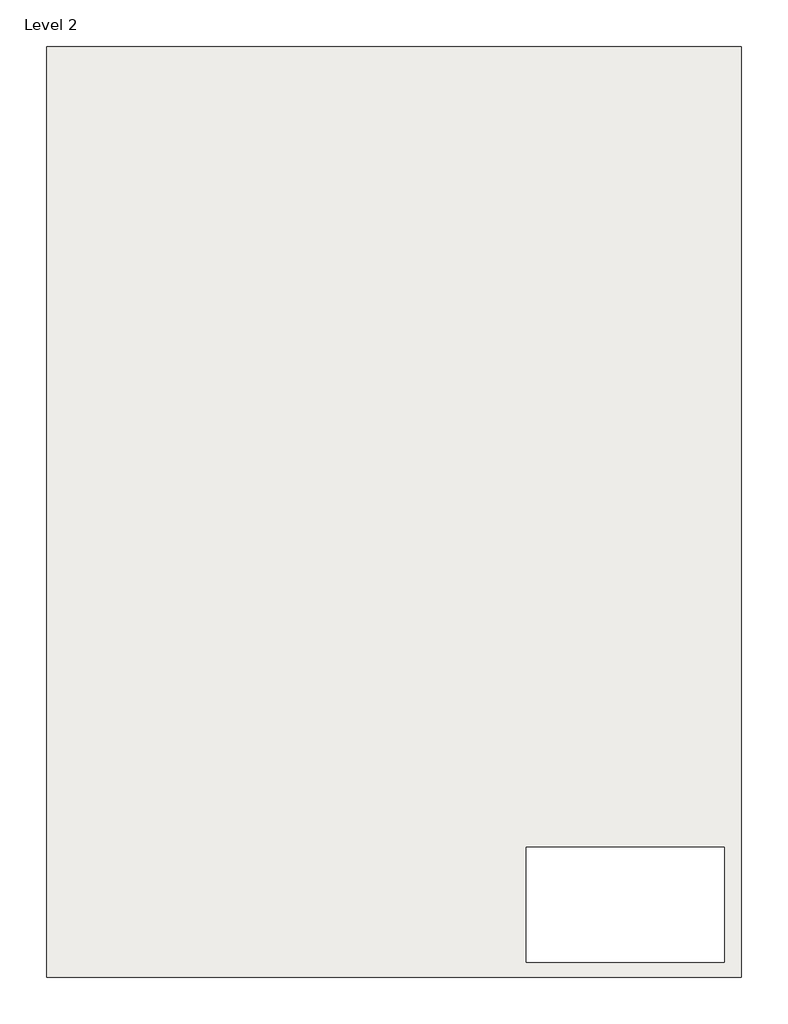
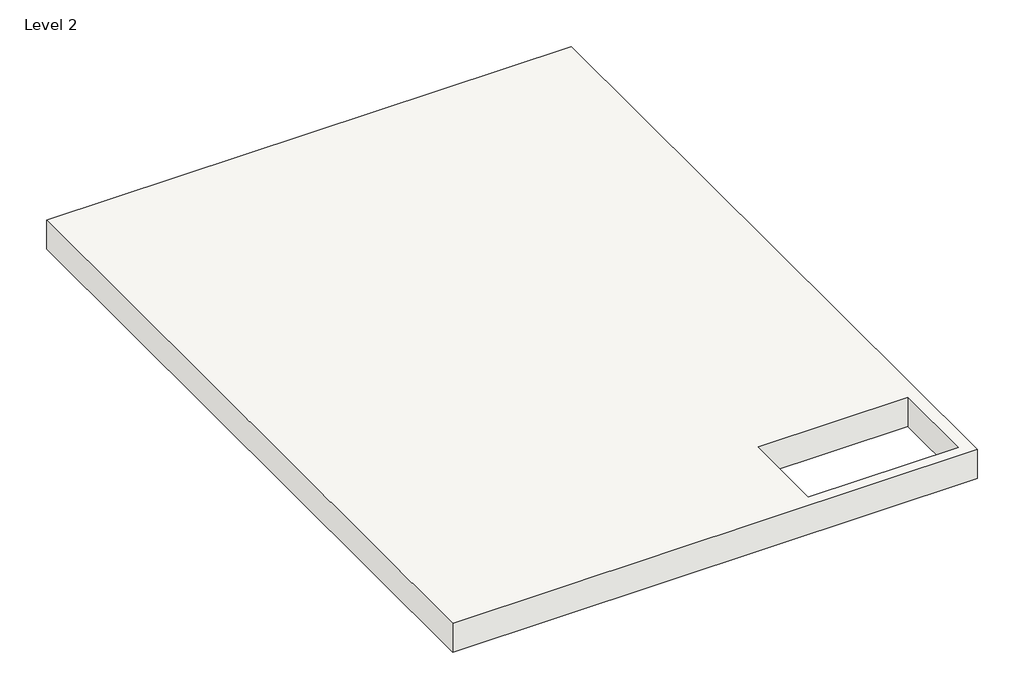
# One storey: 1 roof.
"""IFC4 building model written with IfcOpenShell, lengths in millimetres."""

from ifc_helpers import new_model, si_unit, frame, origin, place, context, project, spatial, polyline, outline, extrude, element, save

model = new_model("IFC4")

# Units and contexts
model_context = context("Model", 3, world=origin())
ifc_project = project(units=[si_unit("LENGTHUNIT", "METRE", prefix="MILLI")], contexts=[model_context])

# Site, building, storey
site = spatial("IfcSite", under=ifc_project)
building = spatial("IfcBuilding", under=site)
storey = spatial("IfcBuildingStorey", under=building, Name="Level 2", Elevation=3048.0)

# Roof
placement = place(None, origin())
element("IfcRoof", 1, ObjectType="Steel Truss - Insulation on Metal Deck - EPDM", at=placement, inside=storey, context=model_context, shape_type="SweptSolid", body=[
    extrude(outline(polyline([(-6658.7041596, 12746.4595092), (2688.4958404, 12746.4595092), (2688.4958404, 224.2595092), (-6658.7041596, 224.2595092), (-6658.7041596, 12746.4595092)]), holes=[polyline([(-206.7168353, 1976.8595092), (-206.7168353, 427.4595092), (2460.2831647, 427.4595092), (2460.2831647, 1976.8595092), (-206.7168353, 1976.8595092)])]), frame((0.0, 0.0, 3048.0), z_axis=(0.0, 0.0, 1.0), x_axis=(1.0, 0.0, 0.0)), (0.0, 0.0, 1.0), 546.1),
])

save(model, "model.ifc")

# Revit data of these elements
# Type "Steel Truss - Insulation on Metal Deck - EPDM"
#   Assembly Code = "B1020"
#   Layers, outside or top first: 0' - 0 1/4" "Roofing, EPDM Membrane" (function 4); 0' - 5" "Rigid insulation" (function 3); 0' - 0 1/4" "Metal Deck" (function 1); 1' - 4" "Structure, Steel Bar Joist Layer" (function 1)
# Element 1 (IfcRoof, "Steel Truss - Insulation on Metal Deck - EPDM")
#   built-in parameter 1001705 = 11.7917 (stored number, unit not read)
#   built-in parameter 1001710 = 33615
#   Phase Created = New Construction
#   Materials on its faces: "Structure, Steel Bar Joist Layer", "Roofing, EPDM Membrane"
# Materials
#   "Roofing, EPDM Membrane": class "Generic", colour RGB 127 127 127, transparency 0, Description = "EPDM roof membrane", Cost = 0
#   "Rigid insulation": class "Generic", colour RGB 127 127 127, transparency 0, Description = "Rigid foam insulation board", Cost = 0
#   "Metal Deck": class "Metal", colour RGB 199 199 199, transparency 0, Description = "Steel, mill finish", Cost = 0
#   "Structure, Steel Bar Joist Layer": class "Metal", colour RGB 127 127 127, transparency 0, Description = "Bar joists, thermal airspace", Cost = 0
